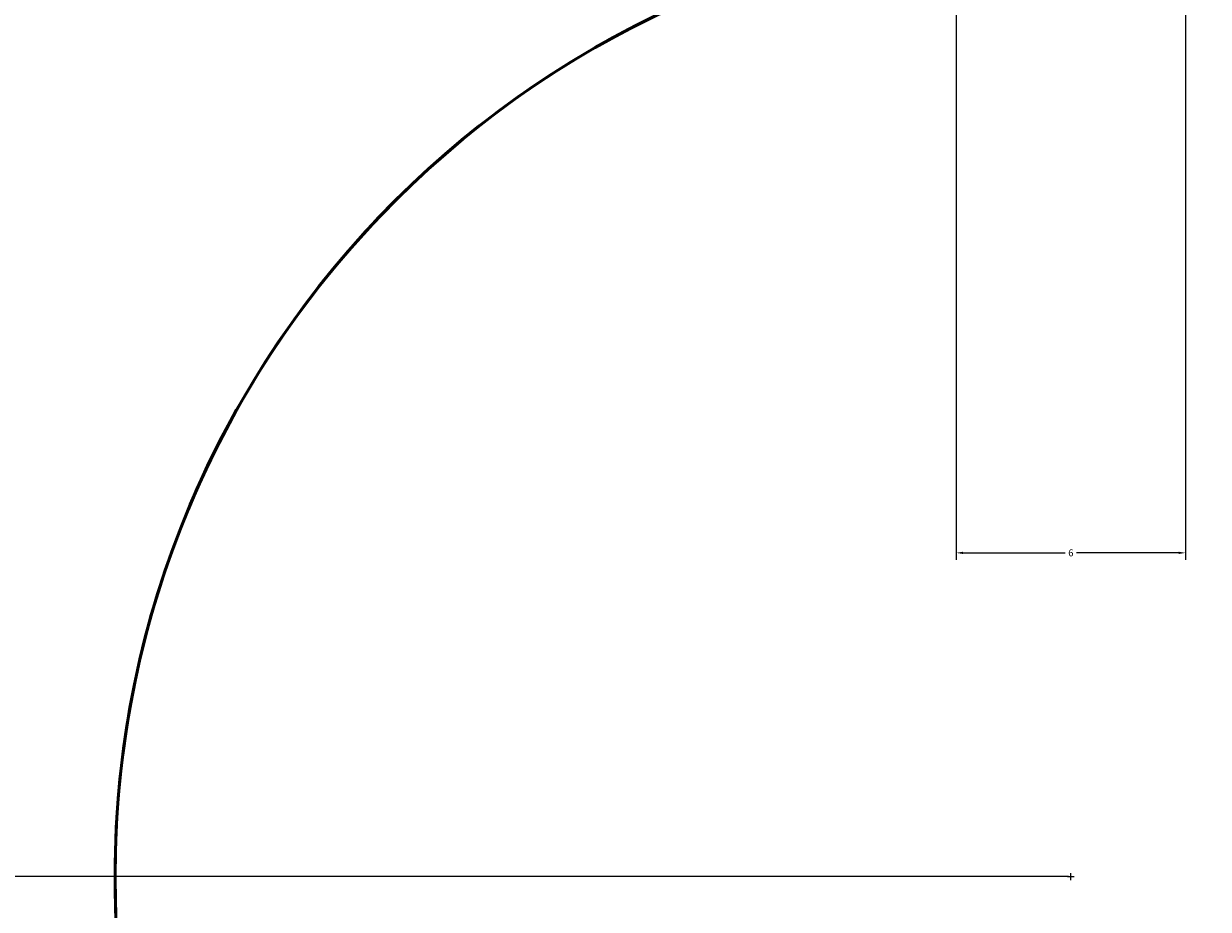
# Model space of a CAD drawing. Units: inches. Extents: x -99 to 284, y -92 to 134.
# Tile 4 of 16: x 5 to 36, y 14 to 37. Entities that reach past the tile are written whole.
import ezdxf

# ---------------------------------------------------------------- set-up
doc = ezdxf.new("R2010")
doc.units = ezdxf.units.IN
doc.header["$MEASUREMENT"] = 0
doc.layers.add('M-DIMS', color=2, linetype='Continuous', lineweight=18)
doc.layers.add('M-OUTL', color=7, linetype='Continuous', lineweight=50)
doc.styles.get("Standard").update_dxf_attribs({"font": 'arial.ttf'})
doc.dimstyles.get("Standard").update_dxf_attribs({"dimtxt": 0.18, "dimasz": 0.18, "dimexe": 0.18, "dimexo": 0.0625, "dimgap": 0.09, "dimtad": 0, "dimtih": 1, "dimtoh": 1, "dimdec": 4, "dimzin": 0, "dimdsep": 46, "dimtxsty": 'Standard', "dimcen": 0.09, "dimadec": 0, "dimazin": 0, "dimtfac": 1, "dimtdec": 4, "dimtofl": 0, "dimtmove": 0, "dimatfit": 3, "dimfxl": 1, "dimtolj": 1, "dimtzin": 0, "dimarcsym": 0})

# ---------------------------------------------------------------- blocks, each defined once
blk = doc.blocks.new('*D3')
at = {"layer": 'Defpoints', "color": 0, "transparency": 16777216}
for p in [(28.976, 39.673), (34.976, 39.673), (28.976, 23.323)]:
    blk.add_point(p, dxfattribs=at)
at = {"layer": 'M-DIMS', "color": 0, "lineweight": -2, "transparency": 16777216}
for p, q in [((28.976, 39.611), (28.976, 23.143)), ((34.976, 39.611), (34.976, 23.143)), ((29.156, 23.323), (31.827, 23.323)), ((34.796, 23.323), (32.126, 23.323))]:
    blk.add_line(p, q, dxfattribs=at)
at = {"layer": 'M-DIMS', "color": 0, "transparency": 16777216}
for points in [[(29.156, 23.353), (29.156, 23.293), (28.976, 23.323)], [(34.796, 23.353), (34.796, 23.293), (34.976, 23.323)]]:
    blk.add_solid(points, dxfattribs=at)
at = {"layer": 'M-DIMS', "color": 0, "transparency": 16777216, "insert": (31.976, 23.323), "char_height": 0.18, "attachment_point": 5}
blk.add_mtext('\\A1;6', dxfattribs=at)
blk = doc.blocks.new('*D9')
at = {"layer": 'Defpoints', "color": 0, "transparency": 16777216}
for p in [(26.771, 58.303), (-73.374, 14.854), (31.976, 14.854)]:
    blk.add_point(p, dxfattribs=at)
at = {"layer": 'M-DIMS', "color": 0, "lineweight": -2, "transparency": 16777216}
for p, q in [((26.709, 58.303), (-73.554, 58.303)), ((-73.374, 58.123), (-73.374, 36.761)), ((-73.374, 15.034), (-73.374, 36.397)), ((31.914, 14.854), (-73.554, 14.854))]:
    blk.add_line(p, q, dxfattribs=at)
at = {"layer": 'M-DIMS', "color": 0, "transparency": 16777216}
for points in [[(-73.404, 58.123), (-73.344, 58.123), (-73.374, 58.303)], [(-73.404, 15.034), (-73.344, 15.034), (-73.374, 14.854)]]:
    blk.add_solid(points, dxfattribs=at)
at = {"layer": 'M-DIMS', "color": 0, "transparency": 16777216, "insert": (-73.374, 36.579), "char_height": 0.18, "attachment_point": 5}
blk.add_mtext('\\A1;43.45', dxfattribs=at)
blk = doc.blocks.new('*D19')
at = {"layer": 'Defpoints', "color": 0, "transparency": 16777216}
for p in [(112.982, 51.721), (-49.029, -22.013)]:
    blk.add_point(p, dxfattribs=at)
at = {"layer": 'M-DIMS', "color": 0, "lineweight": -2, "transparency": 16777216}
for p, q in [((31.976, 14.764), (31.976, 14.944)), ((31.886, 14.854), (32.066, 14.854)), ((-97.632, -44.133), (-49.192, -22.088)), ((-97.812, -44.133), (-97.632, -44.133))]:
    blk.add_line(p, q, dxfattribs=at)
at = {"layer": 'M-DIMS', "color": 0, "transparency": 16777216}
blk.add_solid([(-49.205, -22.06), (-49.18, -22.115), (-49.029, -22.013)], dxfattribs=at)
at = {"layer": 'M-DIMS', "color": 0, "transparency": 16777216, "insert": (-98.199, -44.133), "char_height": 0.18, "attachment_point": 5}
blk.add_mtext('\\A1;∅178', dxfattribs=at)
blk = doc.blocks.new('*D20')
at = {"layer": 'Defpoints', "color": 0, "transparency": 16777216}
for p in [(-35.23, 65.245), (99.183, -35.537)]:
    blk.add_point(p, dxfattribs=at)
at = {"layer": 'M-DIMS', "color": 0, "lineweight": -2, "transparency": 16777216}
for p, q in [((31.976, 14.764), (31.976, 14.944)), ((31.886, 14.854), (32.066, 14.854)), ((139.507, -65.772), (99.327, -35.645)), ((139.687, -65.772), (139.507, -65.772))]:
    blk.add_line(p, q, dxfattribs=at)
at = {"layer": 'M-DIMS', "color": 0, "transparency": 16777216}
blk.add_solid([(99.345, -35.621), (99.309, -35.669), (99.183, -35.537)], dxfattribs=at)
at = {"layer": 'M-DIMS', "color": 0, "transparency": 16777216, "insert": (140.074, -65.772), "char_height": 0.18, "attachment_point": 5}
blk.add_mtext('\\A1;∅168', dxfattribs=at)
blk = doc.blocks.new('*D21')
at = {"layer": 'Defpoints', "color": 0, "transparency": 16777216}
for p in [(19.926, 36.758), (44.027, -7.05)]:
    blk.add_point(p, dxfattribs=at)
at = {"layer": 'M-DIMS', "color": 0, "lineweight": -2, "transparency": 16777216}
for p, q in [((31.976, 14.764), (31.976, 14.944)), ((31.886, 14.854), (32.066, 14.854)), ((51.258, -20.192), (44.114, -7.208)), ((51.438, -20.192), (51.258, -20.192))]:
    blk.add_line(p, q, dxfattribs=at)
at = {"layer": 'M-DIMS', "color": 0, "transparency": 16777216}
blk.add_solid([(44.14, -7.193), (44.088, -7.222), (44.027, -7.05)], dxfattribs=at)
at = {"layer": 'M-DIMS', "color": 0, "transparency": 16777216, "insert": (51.755, -20.192), "char_height": 0.18, "attachment_point": 5}
blk.add_mtext('\\A1;∅50', dxfattribs=at)
blk = doc.blocks.new('*D22')
at = {"layer": 'Defpoints', "color": 0, "transparency": 16777216}
for p in [(39, 89.203), (31.976, 14.854)]:
    blk.add_point(p, dxfattribs=at)
at = {"layer": 'M-DIMS', "color": 0, "lineweight": -2, "transparency": 16777216}
for p, q in [((43.215, 133.813), (39.017, 89.383)), ((43.395, 133.813), (43.215, 133.813)), ((31.976, 14.764), (31.976, 14.944)), ((31.886, 14.854), (32.066, 14.854))]:
    blk.add_line(p, q, dxfattribs=at)
at = {"layer": 'M-DIMS', "color": 0, "transparency": 16777216}
blk.add_solid([(38.987, 89.385), (39.047, 89.38), (39, 89.203)], dxfattribs=at)
at = {"layer": 'M-DIMS', "color": 0, "transparency": 16777216, "insert": (44.068, 133.813), "char_height": 0.18, "attachment_point": 5}
blk.add_mtext('\\A1;5X R74.68', dxfattribs=at)

msp = doc.modelspace()

# ---------------------------------------------------------------- linework, layer by layer
at = {"layer": 'M-OUTL'}
for radius in [89, 84, 25]:
    msp.add_circle((31.9765, 14.8539), radius, dxfattribs=at)
msp.add_arc((31.9765, 14.8539), 25, 96.8921, 83.1079, dxfattribs=at)

# ---------------------------------------------------------------- dimensions: what is measured, and where the dimension line sits
at = {"layer": 'M-DIMS'}
dim = msp.add_radius_dim(center=(31.9765, 14.8539), mpoint=(39.0003, 89.2035), text='5X <>', dimstyle='Standard', override={"dimdec": 2, "dimlfac": 1, "dimrnd": 0, "dimzin": 0, "dimdsep": 46, "dimlunit": 2}, dxfattribs=at)
dim.commit()
dim.dimension.update_dxf_attribs({"geometry": '*D22', "text_midpoint": (44.068, 133.8132), "dimtype": 164})
for p1, p2, picture, middle in [((-35.2301, 65.2451), (99.1831, -35.5373), '*D20', (140.074, -65.772)), ((112.9816, 51.7208), (-49.0286, -22.013), '*D19', (-98.1987, -44.1332)), ((19.9255, 36.7577), (44.0274, -7.0499), '*D21', (51.7545, -20.1921))]:
    dim = msp.add_diameter_dim_2p(p1=p1, p2=p2, dimstyle='Standard', override={"dimdec": 0, "dimlfac": 1, "dimrnd": 0, "dimzin": 0, "dimdsep": 46, "dimlunit": 2}, dxfattribs=at)
    dim.commit()
    dim.dimension.update_dxf_attribs({"geometry": picture, "text_midpoint": middle, "dimtype": 163})
for base, p1, p2, angle, override, picture, middle in [((-73.3735, 14.8539), (26.7713, 58.3032), (31.9765, 14.8539), 90, {"dimdec": 2, "dimlfac": 1, "dimrnd": 0, "dimzin": 0, "dimdsep": 46, "dimlunit": 2}, '*D9', (-73.3735, 36.5785)), ((28.9765, 23.3232), (34.9765, 39.6732), (28.9765, 39.6732), 180, {"dimdec": 0, "dimlfac": 1, "dimrnd": 0, "dimzin": 0, "dimdsep": 46, "dimlunit": 2}, '*D3', (31.9765, 23.3232))]:
    dim = msp.add_linear_dim(base=base, p1=p1, p2=p2, angle=angle, dimstyle='Standard', override=override, dxfattribs=at)
    dim.commit()
    dim.dimension.update_dxf_attribs({"geometry": picture, "text_midpoint": middle})

doc.saveas('drawing.dxf')
